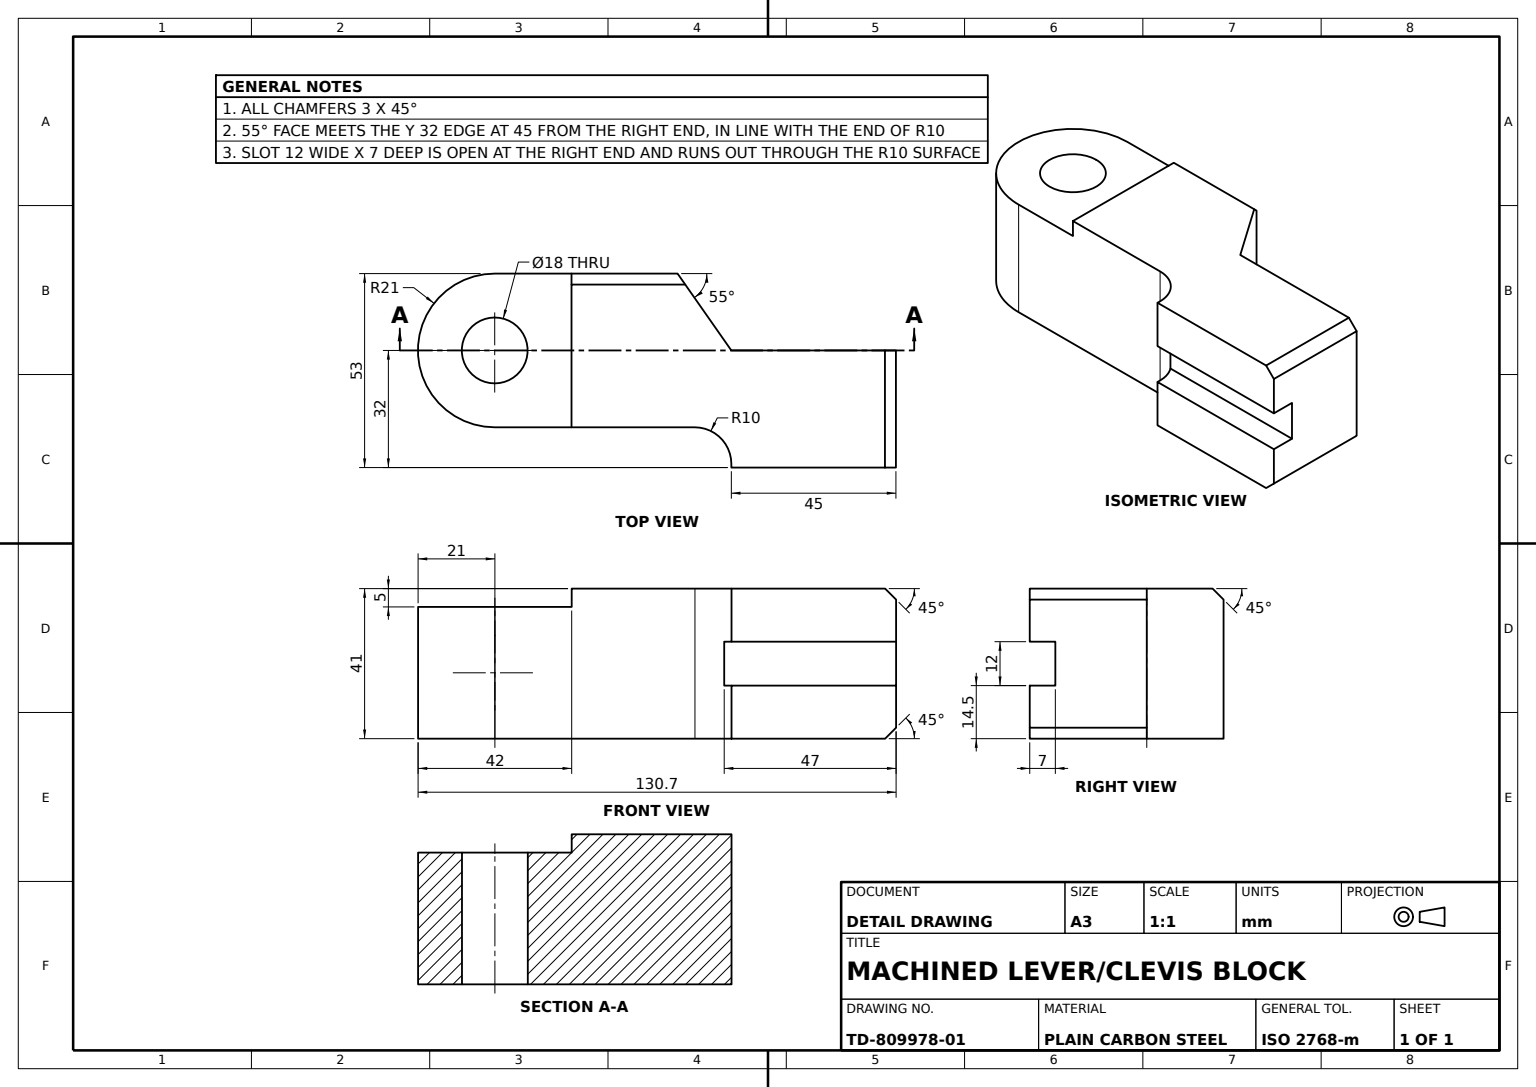
SolidWorks part; units mm, degrees
material "Plain Carbon Steel"
ref_plane "Front Plane" through (0, 0, 0) normal (0, 0, 1) x (1, 0, 0)
ref_plane "Top Plane" through (0, 0, 0) normal (0, 1, 0) x (1, 0, 0)
ref_plane "Right Plane" through (0, 0, 0) normal (1, 0, 0) x (0, 0, -1)
sketch "Link Profile Sketch" plane through (0, 0, 0) normal (0, 1, 0) x (1, 0, 0)
  line L0 (-55, 0) -> (55, 0) construction
  line L3 (9.7044, -32) -> (54.7044, -32)
  line L4 (54.7044, 0) -> (54.7044, -32)
  line L7 (-55, 21) -> (-5, 21)
  line L8 (-55, -21) -> (-0.2956, -21)
  line L9 (-5, 21) -> (9.7044, 0)
  line L10 (54.7044, 0) -> (9.7044, 0)
  line L11 (9.7044, -31) -> (9.7044, -32)
  arc A0 (-55, 21) -> (-55, -21) centre (-55, 0) ccw
  circle A2 centre (-55, 0) radius 9
  arc A3 (9.7044, -31) -> (-0.2956, -21) centre (-0.2956, -31) ccw
  point P0 (0, 0)
  point P8 (0, 0)
  dimension "D1" = 21
  dimension "D3" = 18
  dimension "D11" = 10
  dimension "D2" = 110
  dimension "D4" = 55
  dimension "D5" = 50
  dimension "D6" = 32
  dimension "D7" = 45
  dimension "D8" = 45
  dimension "D9" = 109.7044
  dimension "D10" = 42
extrude "Link Body" add sketch "Link Profile Sketch" along normal mid plane 41
sketch "Eye Recess Sketch" plane through (0, 20.5, 0) normal (0, 1, 0) x (1, 0, 0)
  line L0 (-55, -21) -> (-0.2956, -21) construction
  line L1 (-5, 21) -> (-55, 21) construction
  line L2 (-55, -21) -> (-34, -21)
  line L3 (-34, 21) -> (-55, 21)
  line L4 (-34, 21) -> (-34, -21)
  arc A0 (-55, 21) -> (-55, -21) centre (-55, 0) ccw construction
  arc A1 (-55, 21) -> (-55, -21) centre (-55, 0) ccw
  dimension "D1" = 21
extrude "Eye Recess Cut 5mm" cut sketch "Eye Recess Sketch" against normal blind 5
sketch "Slot Sketch" plane through (54.7044, 0, 0) normal (1, 0, 0) x (0, 0, -1)
  line L0 (-32, 20.5) -> (-32, -20.5) construction
  line L1 (-39, 6) -> (-25, 6)
  line L2 (-39, 6) -> (-39, -6)
  line L3 (-39, -6) -> (-25, -6)
  line L4 (-25, 6) -> (-25, -6)
  line L5 (-39, 6) -> (-25, -6) construction
  line L6 (-39, -6) -> (-25, 6) construction
  point P0 (-32, 0)
  dimension "D1" = 14
  dimension "D2" = 12
extrude "Slot Cut 14x12" cut sketch "Slot Sketch" against normal blind 75
chamfer "End Chamfer 3mm" distance 3 angle 45 3 edges at (54.7044, -20.5, 16) (54.7044, 20.5, 16) (-19.5, 20.5, -21)
